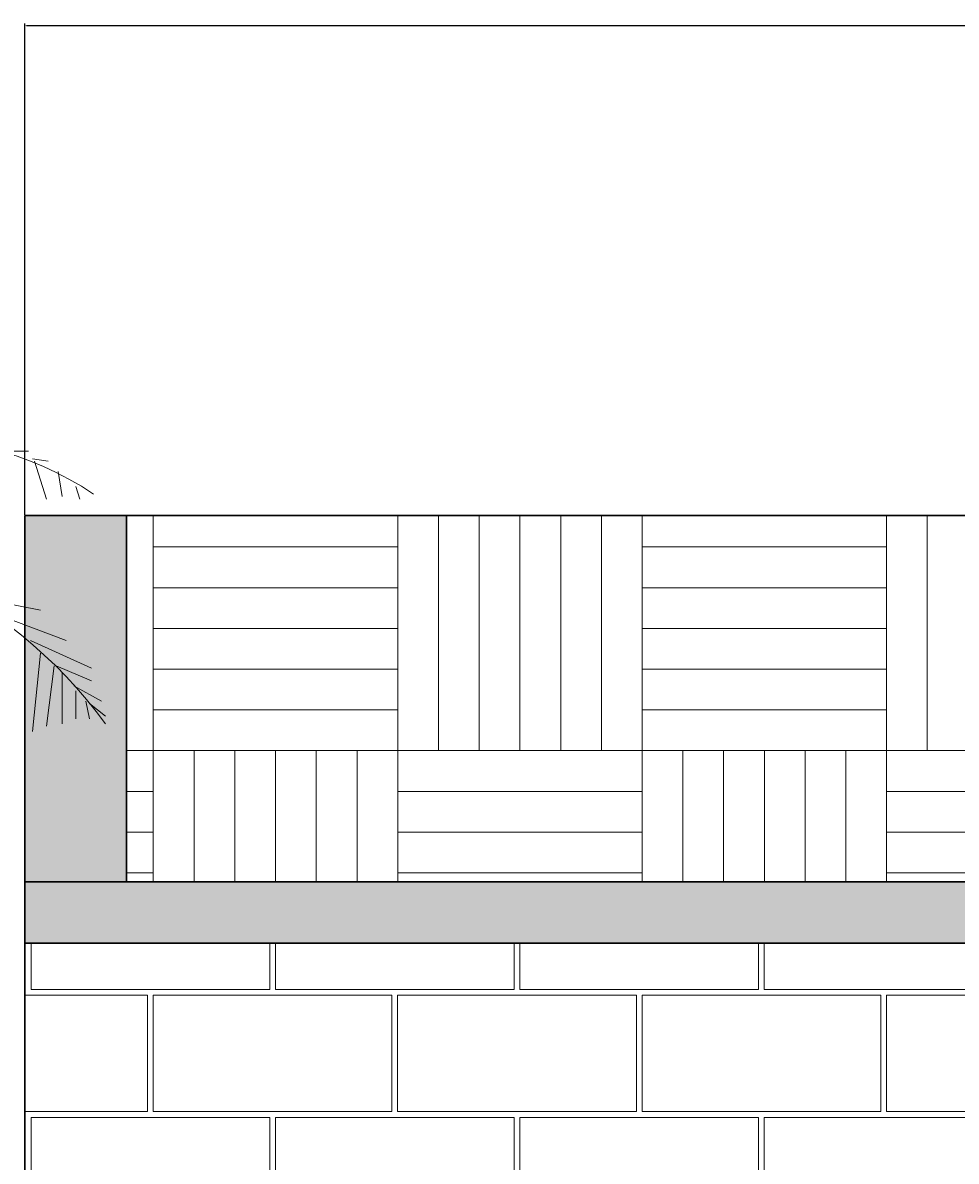
# Model space of a CAD drawing. Units: inches. Extents: x -301 to 715, y -607 to 364.
# Tile 137 of 141: x 254 to 345, y -391 to -279. Entities that reach past the tile are written whole.
import ezdxf

# ---------------------------------------------------------------- set-up
doc = ezdxf.new("R2010")
doc.units = ezdxf.units.IN
doc.header["$MEASUREMENT"] = 0
for name, color, linetype, lineweight in [('A-ANNO-DIMS', 2, 'Continuous', 18), ('A-ELEV', 220, 'Continuous', 30), ('A-ELEV-PATT', 4, 'Continuous', 13), ('L-PLNT', 94, 'Continuous', 13)]:
    doc.layers.add(name, color=color, linetype=linetype, lineweight=lineweight)
doc.styles.get("Standard").update_dxf_attribs({"font": 'arial.ttf'})
doc.dimstyles.get("Standard").update_dxf_attribs({"dimtxt": 0.18, "dimasz": 0.18, "dimexe": 0.18, "dimexo": 0.0625, "dimgap": 0.09, "dimtad": 0, "dimtih": 1, "dimtoh": 1, "dimdec": 1, "dimzin": 0, "dimdsep": 46, "dimlunit": 4, "dimtxsty": 'Standard', "dimcen": 0.09, "dimclrd": 3, "dimclre": 4, "dimclrt": 6, "dimadec": 0, "dimazin": 0, "dimtfac": 1, "dimtdec": 1, "dimtofl": 0, "dimtmove": 0, "dimatfit": 3, "dimfxl": 1, "dimtfill": 2, "dimtfillclr": 51, "dimtolj": 1, "dimtzin": 0, "dimarcsym": 0})

# ---------------------------------------------------------------- blocks, each defined once
blk = doc.blocks.new('*U34')
for p, q in [((32.512, 186.299), (35.218, 186.299)), ((35.605, 185.556), (37.151, 185.308)), ((35.798, 185.308), (36.958, 181.591)), ((38.118, 184.317), (38.504, 181.838)), ((39.857, 182.83), (40.244, 181.591)), ((28.839, 172.174), (36.378, 170.687)), ((30.966, 170.687), (38.891, 167.713)), ((35.412, 167.713), (41.404, 164.988)), ((36.378, 166.474), (35.605, 158.792)), ((37.731, 165.235), (36.958, 159.288)), ((37.924, 165.235), (41.404, 163.749)), ((38.504, 164.492), (38.504, 159.536)), ((39.664, 163.253), (42.37, 161.766)), ((39.857, 162.757), (39.857, 160.031)), ((40.824, 161.766), (41.21, 160.031)), ((41.21, 161.518), (42.757, 160.279))]:
    blk.add_line(p, q)
for centre, radius, start, end in [((23.687, 155.341), 32.188, 56.19272, 134.3213), ((5.828, 132.718), 45.639, 35.98777, 95.82273)]:
    blk.add_arc(centre, radius, start, end)
blk = doc.blocks.new('*D192')
at = {"layer": 'A-ANNO-DIMS', "color": 4, "lineweight": -2, "transparency": 16777216}
for p, q in [((254.02, -327.49), (254.02, -279.27)), ((591.52, -327.49), (591.52, -279.27))]:
    blk.add_line(p, q, dxfattribs=at)
at = {"layer": 'A-ANNO-DIMS', "color": 3, "lineweight": -2, "transparency": 16777216}
for p, q in [((254.2, -279.45), (422.16, -279.45)), ((591.34, -279.45), (423.38, -279.45))]:
    blk.add_line(p, q, dxfattribs=at)
at = {"layer": 'A-ANNO-DIMS', "color": 3, "transparency": 16777216}
for points in [[(254.2, -279.42), (254.2, -279.48), (254.02, -279.45)], [(591.34, -279.42), (591.34, -279.48), (591.52, -279.45)]]:
    blk.add_solid(points, dxfattribs=at)
at = {"layer": 'Defpoints', "color": 0, "transparency": 16777216}
for p in [(591.52, -279.45), (254.02, -327.55), (591.52, -327.55)]:
    blk.add_point(p, dxfattribs=at)
at = {"layer": 'A-ANNO-DIMS', "color": 6, "transparency": 16777216, "insert": (422.77, -279.45), "char_height": 0.18, "attachment_point": 5, "bg_fill": 1, "box_fill_scale": 1.25, "bg_fill_color": 51, "bg_fill_transparency": 0}
blk.add_mtext('\\A1;28\'-1 1/2"', dxfattribs=at)

msp = doc.modelspace()

# ---------------------------------------------------------------- hatches: boundary and pattern name
at = {"layer": 'A-ELEV-PATT'}
h = msp.add_hatch(dxfattribs=at)
h.set_pattern_fill('AR-RROOF', color=256, scale=2)
h.set_pattern_definition([(0, (458.6211, 9.3248), (4.4, 2), [30, -4, 10, -2]), (0, (461.281, 10.3248), (-2, 2.66), [6, -0.66, 12, -1.5]), (0, (459.6211, 11.0248), (10.4, 1.34), [16, -2.8, 8, -2])])
h.paths.add_polyline_path([(254.02, -363.55), (264.02, -363.55), (264.02, -327.55), (254.02, -327.55)])
h.paths.add_polyline_path([(591.52, -327.55), (581.52, -327.55), (581.52, -363.55), (591.52, -363.55)])
h = msp.add_hatch(dxfattribs=at)
h.set_pattern_fill('AR-PARQ1', color=256, scale=2)
h.set_pattern_definition([(90, (458.62, 9.325), (-24, 24), [24, -24]), (90, (462.62, 9.325), (-24, 24), [24, -24]), (90, (466.62, 9.325), (-24, 24), [24, -24]), (90, (470.62, 9.325), (-24, 24), [24, -24]), (90, (474.62, 9.325), (-24, 24), [24, -24]), (90, (478.62, 9.325), (-24, 24), [24, -24]), (90, (482.62, 9.325), (-24, 24), [24, -24]), (0, (458.62, 33.325), (24, -24), [24, -24]), (0, (458.62, 37.325), (24, -24), [24, -24]), (0, (458.62, 41.325), (24, -24), [24, -24]), (0, (458.62, 45.325), (24, -24), [24, -24]), (0, (458.62, 49.325), (24, -24), [24, -24]), (0, (458.62, 53.325), (24, -24), [24, -24]), (0, (458.62, 57.325), (24, -24), [24, -24])])
h.paths.add_polyline_path([(264.02, -327.55), (264.02, -363.55), (581.52, -363.55), (581.52, -327.55)])
h = msp.add_hatch(color=256, dxfattribs=at)
h.dxf.hatch_style = 1
h.paths.add_polyline_path([(591.52, -363.55), (254.02, -363.55), (254.02, -369.55), (591.52, -369.55)])
h.paths.add_polyline_path([(461.02, -393.55), (413.02, -393.55), (413.02, -489.55), (461.02, -489.55)])
h.paths.add_polyline_path([(456.02, -398.55), (456.02, -484.55), (418.02, -484.55), (418.02, -398.55)], flags=16)
h.paths.add_polyline_path([(546.77, -393.55), (496.77, -393.55), (496.77, -441.55), (546.77, -441.55)])
h.paths.add_polyline_path([(501.77, -398.55), (541.77, -398.55), (541.77, -436.55), (501.77, -436.55)], flags=16)
h.paths.add_polyline_path([(360.02, -393.55), (310.02, -393.55), (310.02, -441.55), (360.02, -441.55)])
h.paths.add_polyline_path([(355.02, -398.55), (355.02, -436.55), (315.02, -436.55), (315.02, -398.55)], flags=16)
h = msp.add_hatch(dxfattribs=at)
h.set_pattern_fill('AR-B816C', color=256, scale=1.5)
h.set_pattern_definition([(0, (458.621, 9.325), (12, 12), [23.4375, -0.5625]), (0, (446.621, 9.887), (12, 12), [23.4375, -0.5625]), (90, (458.621, 9.325), (-12, 12), [-12.5625, 11.4375]), (90, (458.059, 9.325), (-12, 12), [-12.5625, 11.4375])])
h.paths.add_polyline_path([(254.02, -489.55), (413.02, -489.55), (413.02, -393.55), (461.02, -393.55), (461.02, -489.55), (591.52, -489.55), (591.52, -369.55), (254.02, -369.55)])
h.paths.add_polyline_path([(310.02, -393.55), (360.02, -393.55), (360.02, -441.55), (310.02, -441.55)], flags=16)
h.paths.add_polyline_path([(315.02, -398.55), (355.02, -398.55), (355.02, -436.55), (315.02, -436.55)], flags=0)
h.paths.add_polyline_path([(496.77, -393.55), (546.77, -393.55), (546.77, -441.55), (496.77, -441.55)], flags=16)
h.paths.add_polyline_path([(501.77, -398.55), (541.77, -398.55), (541.77, -436.55), (501.77, -436.55)], flags=0)

# ---------------------------------------------------------------- linework, layer by layer
at = {"layer": 'A-ELEV'}
for p, q in [((254.02, -327.55), (591.52, -327.55)), ((254.02, -327.55), (264.02, -327.55)), ((264.02, -327.55), (264.02, -363.55)), ((254.02, -363.55), (591.52, -363.55)), ((254.02, -369.55), (591.52, -369.55))]:
    msp.add_line(p, q, dxfattribs=at)
for points in [[(254.02, -327.55), (591.52, -327.55), (591.52, -363.55), (254.02, -363.55)], [(254.02, -363.55), (591.52, -363.55), (591.52, -369.55), (254.02, -369.55)], [(254.02, -369.55), (591.52, -369.55), (591.52, -489.55), (254.02, -489.55)]]:
    msp.add_lwpolyline(points, close=True, dxfattribs=at)

# ---------------------------------------------------------------- block references
at = {"layer": 'L-PLNT'}
msp.add_blockref('*U34', (219.18, -507.55), dxfattribs=at)

# ---------------------------------------------------------------- dimensions: what is measured, and where the dimension line sits
at = {"layer": 'A-ANNO-DIMS'}
dim = msp.add_linear_dim(base=(591.52, -279.45), p1=(254.02, -327.55), p2=(591.52, -327.55), dimstyle='Standard', override={"dimdec": 1, "dimlfac": 1, "dimrnd": 0, "dimzin": 1, "dimdsep": 46, "dimlunit": 4, "dimfrac": 2}, dxfattribs=at)
dim.commit()
dim.dimension.update_dxf_attribs({"geometry": '*D192', "text_midpoint": (422.77, -279.45)})

doc.saveas('drawing.dxf')
